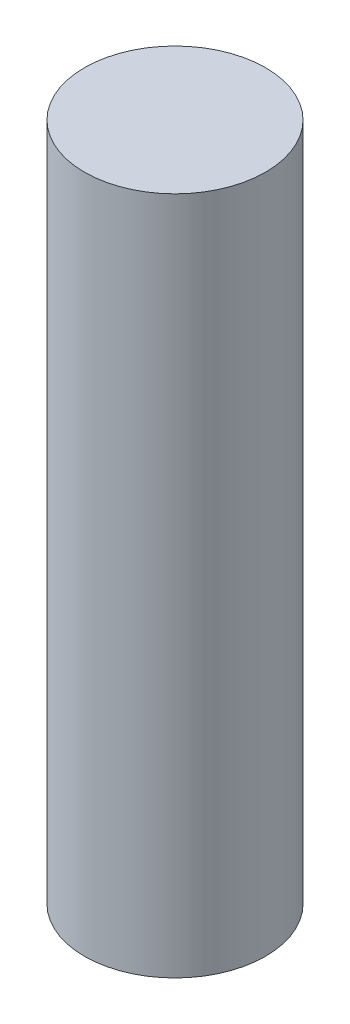
SolidWorks part; units mm, degrees
material "Plain Carbon Steel"
ref_plane "Front Plane" through (0, 0, 0) normal (0, 0, 1) x (1, 0, 0)
ref_plane "Top Plane" through (0, 0, 0) normal (0, 1, 0) x (1, 0, 0)
ref_plane "Right Plane" through (0, 0, 0) normal (1, 0, 0) x (0, 0, -1)
sketch "Shank Profile Ø12" plane through (0, 0, 0) normal (0, 1, 0) x (1, 0, 0)
  circle A0 centre (0, 0) radius 6
  dimension "D1" = 12
extrude "Shank Ø12x45" add sketch "Shank Profile Ø12" along normal mid plane 45
